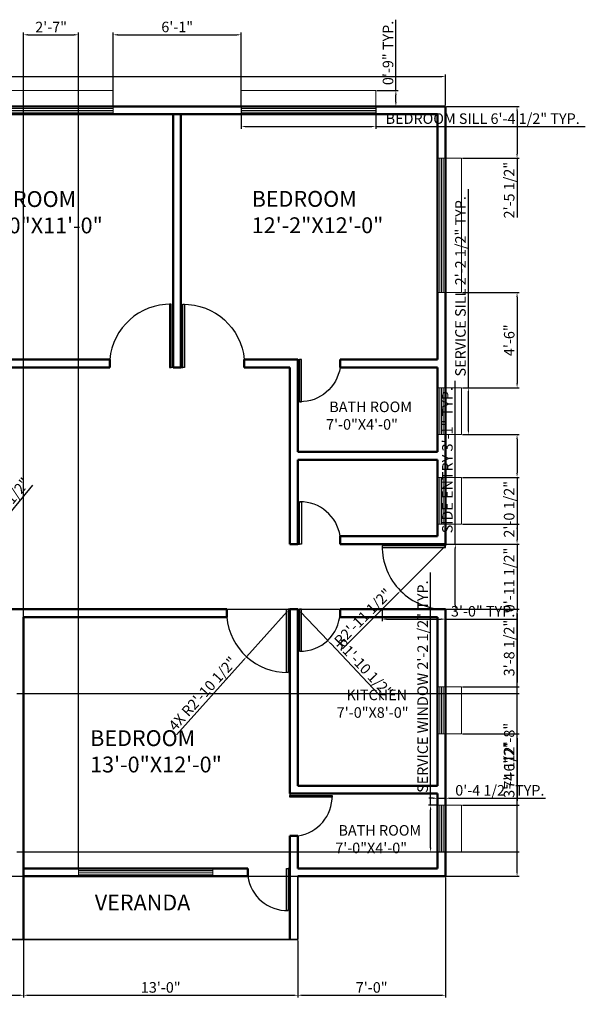
# Model space of a CAD drawing. Units: inches. Extents: x 2373 to 3112, y 1710 to 2270.
# Tile 2 of 2: x 2790 to 3112, y 1710 to 2270. Entities that reach past the tile are written whole.
import ezdxf

# ---------------------------------------------------------------- set-up
doc = ezdxf.new("R2010")
doc.units = ezdxf.units.IN
doc.layers.add('A-ANNO-DIMS', color=7, linetype='Continuous', lineweight=18)
doc.layers.add('A-AREA-IDEN', color=7, linetype='Continuous', lineweight=25)
for name, color, linetype, lineweight, true_color in [('A-DOOR', 114, 'Continuous', 25, 0x139b48), ('A-FLOR', 114, 'Continuous', 35, 0x139b48), ('A-GLAZ', 31, 'Continuous', 18, 0xfecc66), ('A-GLAZ-SILL', 30, 'Continuous', 18, 0xf8991e), ('A-WALL', 114, 'Continuous', 50, 0x139b48)]:
    doc.layers.add(name, color=color, linetype=linetype, lineweight=lineweight, true_color=true_color)
doc.styles.get("Standard").update_dxf_attribs({"font": 'arial.ttf'})
doc.dimstyles.new('ISO-25', dxfattribs={"dimtxt": 6, "dimasz": 2.5, "dimexe": 1.25, "dimexo": 0.625, "dimtad": 1, "dimdec": 1, "dimlunit": 3, "dimtxsty": 'Standard', "dimcen": 2.5, "dimadec": 0, "dimazin": 0, "dimtfac": 1, "dimtdec": 1, "dimtmove": 0, "dimatfit": 3, "dimfxl": 1, "dimarcsym": 0})

# ---------------------------------------------------------------- blocks, each defined once
blk = doc.blocks.new('*D2')
at = {"layer": 'A-ANNO-DIMS', "color": 0, "lineweight": -2, "transparency": 16777216}
for p, q in [((2426.36, 2221.72), (2426.36, 2239.32)), ((2428.86, 2238.07), (3029.86, 2238.07)), ((3032.36, 2221.72), (3032.36, 2239.32))]:
    blk.add_line(p, q, dxfattribs=at)
at = {"layer": 'A-ANNO-DIMS', "color": 0, "transparency": 16777216}
for points in [[(2428.86, 2238.48), (2428.86, 2237.65), (2426.36, 2238.07)], [(3029.86, 2238.48), (3029.86, 2237.65), (3032.36, 2238.07)]]:
    blk.add_solid(points, dxfattribs=at)
at = {"layer": 'Defpoints', "color": 0, "transparency": 16777216}
for p in [(3032.36, 2238.07), (2426.36, 2221.09), (3032.36, 2221.09)]:
    blk.add_point(p, dxfattribs=at)
at = {"layer": 'A-ANNO-DIMS', "color": 0, "transparency": 16777216, "insert": (2729.36, 2241.76), "char_height": 6, "attachment_point": 5}
blk.add_mtext('50\'-6"', dxfattribs=at)
blk = doc.blocks.new('DOOR-SWING-24IN')
for p, q in [((-2, -24), (-2, 0)), ((-2, 0), (-1, 0)), ((0, 0), (-1, 0)), ((-1, 0), (-1, -24)), ((-1, -24), (-2, -24))]:
    blk.add_line(p, q)
blk.add_arc((-1.5, -1.28), 22.73, 188.1552, 271.2605)
blk = doc.blocks.new('DOOR-SWING-36IN')
for p, q in [((-1, 36), (-2, 36)), ((-2, 36), (-2, 0)), ((-1, 0), (-1, 36)), ((-2, 0), (-1, 0)), ((0, 0), (-1, 0))]:
    blk.add_line(p, q)
blk.add_arc((-1.5, 1.36), 34.64, 89.173, 174.8014)
blk = doc.blocks.new('DOOR-SIDE-ENTRY-36IN')
for p, q in [((0, 0), (0, -1)), ((0, -1), (-36, -1)), ((-36, -1), (-36, -2)), ((-36, -2), (0, -2)), ((0, -2), (0, -1))]:
    blk.add_line(p, q)
blk.add_arc((-0.5, -1.5), 35.5, 179.1931, 270.8069)
blk = doc.blocks.new('WINDOW-BEDROOM')
for p, q in [((0, 0), (0, -4.5)), ((76.46, 0), (0, 0)), ((0, 0), (0, -2.25)), ((76.46, -4.5), (76.46, 0)), ((76.46, -1.25), (0, -1.25)), ((0, -1.25), (0, -2.25)), ((0, -2.25), (76.46, -2.25)), ((0, -2.25), (0, -3.25)), ((0, -3.25), (76.46, -3.25)), ((0, -4.5), (76.46, -4.5)), ((76.46, -2.25), (76.46, -1.25))]:
    blk.add_line(p, q)
blk = doc.blocks.new('WINDOW-SERVICE')
for p, q in [((0, 0), (0, -26.66)), ((4.5, 0), (0, 0)), ((1.25, 0), (1.25, -26.66)), ((2.25, 0), (2.25, -26.66)), ((3.25, -26.66), (3.25, 0)), ((4.5, -26.66), (4.5, 0)), ((4.5, -26.66), (4.5, 0)), ((0, -26.66), (4.5, -26.66))]:
    blk.add_line(p, q)
blk = doc.blocks.new('SILL-SERVICE')
for p, q in [((0, 0), (9, 0)), ((9, 0), (9, -26.66)), ((9, -26.66), (0, -26.66))]:
    blk.add_line(p, q)
blk = doc.blocks.new('SILL-BEDROOM')
for p, q in [((0, 0), (0, 9)), ((0, 9), (76.46, 9)), ((76.46, 9), (76.46, 0))]:
    blk.add_line(p, q)
blk = doc.blocks.new('*D16')
at = {"layer": 'A-ANNO-DIMS', "color": 0, "lineweight": -2, "transparency": 16777216}
for p, q in [((3037.93, 1972.09), (3037.93, 2065.02)), ((3032.99, 1972.09), (3039.18, 1972.09)), ((3037.93, 1937.46), (3037.93, 1969.59)), ((3032.99, 1934.96), (3039.18, 1934.96))]:
    blk.add_line(p, q, dxfattribs=at)
at = {"layer": 'A-ANNO-DIMS', "color": 0, "transparency": 16777216}
for points in [[(3037.52, 1969.59), (3038.35, 1969.59), (3037.93, 1972.09)], [(3037.52, 1937.46), (3038.35, 1937.46), (3037.93, 1934.96)]]:
    blk.add_solid(points, dxfattribs=at)
at = {"layer": 'Defpoints', "color": 0, "transparency": 16777216}
for p in [(3032.36, 1972.09), (3037.93, 1972.09), (3032.36, 1934.96)]:
    blk.add_point(p, dxfattribs=at)
at = {"layer": 'A-ANNO-DIMS', "color": 0, "transparency": 16777216, "insert": (3034.2, 2019.81), "char_height": 6, "attachment_point": 5, "rotation": 90}
blk.add_mtext('SIDE ENTRY 3\'-1" TYP.', dxfattribs=at)
blk = doc.blocks.new('*D17')
at = {"layer": 'A-ANNO-DIMS', "color": 0, "lineweight": -2, "transparency": 16777216}
for p, q in [((2996.23, 1934.33), (2996.23, 1928.14)), ((3032.36, 1934.33), (3032.36, 1928.14)), ((2998.73, 1929.39), (3029.86, 1929.39)), ((3032.36, 1929.39), (3072.68, 1929.39))]:
    blk.add_line(p, q, dxfattribs=at)
at = {"layer": 'A-ANNO-DIMS', "color": 0, "transparency": 16777216}
for points in [[(2998.73, 1929.81), (2998.73, 1928.97), (2996.23, 1929.39)], [(3029.86, 1929.81), (3029.86, 1928.97), (3032.36, 1929.39)]]:
    blk.add_solid(points, dxfattribs=at)
at = {"layer": 'Defpoints', "color": 0, "transparency": 16777216}
for p in [(2996.23, 1934.96), (3032.36, 1934.96), (3032.36, 1929.39)]:
    blk.add_point(p, dxfattribs=at)
at = {"layer": 'A-ANNO-DIMS', "color": 0, "transparency": 16777216, "insert": (3053.77, 1933.08), "char_height": 6, "attachment_point": 5}
blk.add_mtext('3\'-0" TYP.', dxfattribs=at)
blk = doc.blocks.new('*D20')
at = {"layer": 'A-ANNO-DIMS', "color": 0, "lineweight": -2, "transparency": 16777216}
for p, q in [((3023.86, 1823.48), (3023.86, 1955.99)), ((3027.24, 1823.48), (3022.61, 1823.48)), ((3023.86, 1799.32), (3023.86, 1820.98)), ((3027.24, 1796.82), (3022.61, 1796.82))]:
    blk.add_line(p, q, dxfattribs=at)
at = {"layer": 'A-ANNO-DIMS', "color": 0, "transparency": 16777216}
for points in [[(3023.45, 1820.98), (3024.28, 1820.98), (3023.86, 1823.48)], [(3023.45, 1799.32), (3024.28, 1799.32), (3023.86, 1796.82)]]:
    blk.add_solid(points, dxfattribs=at)
at = {"layer": 'Defpoints', "color": 0, "transparency": 16777216}
for p in [(3023.86, 1823.48), (3027.86, 1823.48), (3027.86, 1796.82)]:
    blk.add_point(p, dxfattribs=at)
at = {"layer": 'A-ANNO-DIMS', "color": 0, "transparency": 16777216, "insert": (3020.14, 1890.98), "char_height": 6, "attachment_point": 5, "rotation": 90}
blk.add_mtext('SERVICE WINDOW 2\'-2 1/2" TYP.', dxfattribs=at)
blk = doc.blocks.new('*D21')
at = {"layer": 'A-ANNO-DIMS', "color": 0, "lineweight": -2, "transparency": 16777216}
for p, q in [((3025.36, 1827.48), (3022.86, 1827.48)), ((3027.86, 1824.1), (3027.86, 1828.73)), ((3027.86, 1827.48), (3032.36, 1827.48)), ((3032.36, 1824.1), (3032.36, 1828.73)), ((3034.86, 1827.48), (3089.17, 1827.48))]:
    blk.add_line(p, q, dxfattribs=at)
at = {"layer": 'A-ANNO-DIMS', "color": 0, "transparency": 16777216}
for points in [[(3025.36, 1827.9), (3025.36, 1827.06), (3027.86, 1827.48)], [(3034.86, 1827.9), (3034.86, 1827.06), (3032.36, 1827.48)]]:
    blk.add_solid(points, dxfattribs=at)
at = {"layer": 'Defpoints', "color": 0, "transparency": 16777216}
for p in [(3032.36, 1827.48), (3027.86, 1823.48), (3032.36, 1823.48)]:
    blk.add_point(p, dxfattribs=at)
at = {"layer": 'A-ANNO-DIMS', "color": 0, "transparency": 16777216, "insert": (3063.27, 1831.21), "char_height": 6, "attachment_point": 5}
blk.add_mtext('0\'-4 1/2" TYP.', dxfattribs=at)
blk = doc.blocks.new('*D22')
at = {"layer": 'A-ANNO-DIMS', "color": 0, "lineweight": -2, "transparency": 16777216}
for p, q in [((3045.36, 2061), (3045.36, 2173.98)), ((3041.99, 2061), (3046.61, 2061)), ((3045.36, 2036.84), (3045.36, 2058.5)), ((3041.99, 2034.34), (3046.61, 2034.34))]:
    blk.add_line(p, q, dxfattribs=at)
at = {"layer": 'A-ANNO-DIMS', "color": 0, "transparency": 16777216}
for points in [[(3044.95, 2058.5), (3045.78, 2058.5), (3045.36, 2061)], [(3044.95, 2036.84), (3045.78, 2036.84), (3045.36, 2034.34)]]:
    blk.add_solid(points, dxfattribs=at)
at = {"layer": 'Defpoints', "color": 0, "transparency": 16777216}
for p in [(3041.36, 2061), (3045.36, 2061), (3041.36, 2034.34)]:
    blk.add_point(p, dxfattribs=at)
at = {"layer": 'A-ANNO-DIMS', "color": 0, "transparency": 16777216, "insert": (3041.64, 2118.74), "char_height": 6, "attachment_point": 5, "rotation": 90}
blk.add_mtext('SERVICE SILL 2\'-2 1/2" TYP.', dxfattribs=at)
blk = doc.blocks.new('*D24')
at = {"layer": 'A-ANNO-DIMS', "color": 0, "lineweight": -2, "transparency": 16777216}
for p, q in [((2916.18, 2220.47), (2916.18, 2208.38)), ((2992.64, 2220.47), (2992.64, 2208.38)), ((2918.68, 2209.63), (2990.14, 2209.63)), ((2992.64, 2209.63), (3111.89, 2209.63))]:
    blk.add_line(p, q, dxfattribs=at)
at = {"layer": 'A-ANNO-DIMS', "color": 0, "transparency": 16777216}
for points in [[(2918.68, 2210.04), (2918.68, 2209.21), (2916.18, 2209.63)], [(2990.14, 2210.04), (2990.14, 2209.21), (2992.64, 2209.63)]]:
    blk.add_solid(points, dxfattribs=at)
at = {"layer": 'Defpoints', "color": 0, "transparency": 16777216}
for p in [(2916.18, 2221.09), (2992.64, 2221.09), (2992.64, 2209.63)]:
    blk.add_point(p, dxfattribs=at)
at = {"layer": 'A-ANNO-DIMS', "color": 0, "transparency": 16777216, "insert": (3053.51, 2213.36), "char_height": 6, "attachment_point": 5}
blk.add_mtext('BEDROOM SILL 6\'-4 1/2" TYP.', dxfattribs=at)
blk = doc.blocks.new('*D25')
at = {"layer": 'A-ANNO-DIMS', "color": 0, "lineweight": -2, "transparency": 16777216}
for p, q in [((3004.11, 2230.09), (3004.11, 2270.42)), ((2993.26, 2230.09), (3005.36, 2230.09)), ((3004.11, 2223.59), (3004.11, 2227.59)), ((2993.26, 2221.09), (3005.36, 2221.09))]:
    blk.add_line(p, q, dxfattribs=at)
at = {"layer": 'A-ANNO-DIMS', "color": 0, "transparency": 16777216}
for points in [[(3003.69, 2227.59), (3004.53, 2227.59), (3004.11, 2230.09)], [(3003.69, 2223.59), (3004.53, 2223.59), (3004.11, 2221.09)]]:
    blk.add_solid(points, dxfattribs=at)
at = {"layer": 'Defpoints', "color": 0, "transparency": 16777216}
for p in [(2992.64, 2230.09), (3004.11, 2230.09), (2992.64, 2221.09)]:
    blk.add_point(p, dxfattribs=at)
at = {"layer": 'A-ANNO-DIMS', "color": 0, "transparency": 16777216, "insert": (3000.42, 2251.51), "char_height": 6, "attachment_point": 5, "rotation": 90}
blk.add_mtext('0\'-9" TYP.', dxfattribs=at)
blk = doc.blocks.new('*D31')
at = {"layer": 'A-ANNO-DIMS', "color": 0, "lineweight": -2, "transparency": 16777216}
for p, q in [((2670.86, 1746.47), (2670.86, 1714.14)), ((2792.36, 1746.47), (2792.36, 1714.14)), ((2673.36, 1715.39), (2789.86, 1715.39))]:
    blk.add_line(p, q, dxfattribs=at)
at = {"layer": 'A-ANNO-DIMS', "color": 0, "transparency": 16777216}
for points in [[(2673.36, 1715.81), (2673.36, 1714.97), (2670.86, 1715.39)], [(2789.86, 1715.81), (2789.86, 1714.97), (2792.36, 1715.39)]]:
    blk.add_solid(points, dxfattribs=at)
at = {"layer": 'Defpoints', "color": 0, "transparency": 16777216}
for p in [(2670.86, 1747.09), (2792.36, 1747.09), (2792.36, 1715.39)]:
    blk.add_point(p, dxfattribs=at)
at = {"layer": 'A-ANNO-DIMS', "color": 0, "transparency": 16777216, "insert": (2731.61, 1719.12), "char_height": 6, "attachment_point": 5}
blk.add_mtext('10\'-1 1/2"', dxfattribs=at)
blk = doc.blocks.new('*D32')
at = {"layer": 'A-ANNO-DIMS', "color": 0, "lineweight": -2, "transparency": 16777216}
for p, q in [((2792.36, 1746.47), (2792.36, 1714.14)), ((2948.36, 1746.47), (2948.36, 1714.14)), ((2794.86, 1715.39), (2945.86, 1715.39))]:
    blk.add_line(p, q, dxfattribs=at)
at = {"layer": 'A-ANNO-DIMS', "color": 0, "transparency": 16777216}
for points in [[(2794.86, 1715.81), (2794.86, 1714.97), (2792.36, 1715.39)], [(2945.86, 1715.81), (2945.86, 1714.97), (2948.36, 1715.39)]]:
    blk.add_solid(points, dxfattribs=at)
at = {"layer": 'Defpoints', "color": 0, "transparency": 16777216}
for p in [(2792.36, 1747.09), (2948.36, 1747.09), (2948.36, 1715.39)]:
    blk.add_point(p, dxfattribs=at)
at = {"layer": 'A-ANNO-DIMS', "color": 0, "transparency": 16777216, "insert": (2870.36, 1719.08), "char_height": 6, "attachment_point": 5}
blk.add_mtext('13\'-0"', dxfattribs=at)
blk = doc.blocks.new('*D33')
at = {"layer": 'A-ANNO-DIMS', "color": 0, "lineweight": -2, "transparency": 16777216}
for p, q in [((3032.36, 1782.47), (3032.36, 1714.14)), ((2948.36, 1746.47), (2948.36, 1714.14)), ((2950.86, 1715.39), (3029.86, 1715.39))]:
    blk.add_line(p, q, dxfattribs=at)
at = {"layer": 'A-ANNO-DIMS', "color": 0, "transparency": 16777216}
for points in [[(2950.86, 1715.81), (2950.86, 1714.97), (2948.36, 1715.39)], [(3029.86, 1715.81), (3029.86, 1714.97), (3032.36, 1715.39)]]:
    blk.add_solid(points, dxfattribs=at)
at = {"layer": 'Defpoints', "color": 0, "transparency": 16777216}
for p in [(3032.36, 1783.09), (2948.36, 1747.09), (3032.36, 1715.39)]:
    blk.add_point(p, dxfattribs=at)
at = {"layer": 'A-ANNO-DIMS', "color": 0, "transparency": 16777216, "insert": (2990.36, 1719.08), "char_height": 6, "attachment_point": 5}
blk.add_mtext('7\'-0"', dxfattribs=at)
blk = doc.blocks.new('*D34')
at = {"layer": 'A-ANNO-DIMS', "color": 0, "lineweight": -2, "transparency": 16777216}
for p, q in [((2555.99, 1935.09), (3074.32, 1935.09)), ((3073.07, 1785.59), (3073.07, 1932.59)), ((2571.63, 1783.09), (3074.32, 1783.09))]:
    blk.add_line(p, q, dxfattribs=at)
at = {"layer": 'A-ANNO-DIMS', "color": 0, "transparency": 16777216}
for points in [[(3072.65, 1932.59), (3073.49, 1932.59), (3073.07, 1935.09)], [(3072.65, 1785.59), (3073.49, 1785.59), (3073.07, 1783.09)]]:
    blk.add_solid(points, dxfattribs=at)
at = {"layer": 'Defpoints', "color": 0, "transparency": 16777216}
for p in [(2555.36, 1935.09), (3073.07, 1935.09), (2571, 1783.09)]:
    blk.add_point(p, dxfattribs=at)
at = {"layer": 'A-ANNO-DIMS', "color": 0, "transparency": 16777216, "insert": (3069.38, 1859.09), "char_height": 6, "attachment_point": 5, "rotation": 90}
blk.add_mtext('12\'-8"', dxfattribs=at)
blk = doc.blocks.new('*D38')
at = {"layer": 'A-ANNO-DIMS', "color": 0, "lineweight": -2, "transparency": 16777216}
for p, q in [((2843.26, 2221.72), (2843.26, 2263.07)), ((2845.76, 2261.82), (2913.68, 2261.82)), ((2916.18, 2221.72), (2916.18, 2263.07))]:
    blk.add_line(p, q, dxfattribs=at)
at = {"layer": 'A-ANNO-DIMS', "color": 0, "transparency": 16777216}
for points in [[(2845.76, 2262.24), (2845.76, 2261.4), (2843.26, 2261.82)], [(2913.68, 2262.24), (2913.68, 2261.4), (2916.18, 2261.82)]]:
    blk.add_solid(points, dxfattribs=at)
at = {"layer": 'Defpoints', "color": 0, "transparency": 16777216}
for p in [(2916.18, 2261.82), (2843.26, 2221.09), (2916.18, 2221.09)]:
    blk.add_point(p, dxfattribs=at)
at = {"layer": 'A-ANNO-DIMS', "color": 0, "transparency": 16777216, "insert": (2879.72, 2265.51), "char_height": 6, "attachment_point": 5}
blk.add_mtext('6\'-1"', dxfattribs=at)
blk = doc.blocks.new('*D39')
at = {"layer": 'A-ANNO-DIMS', "color": 0, "lineweight": -2, "transparency": 16777216}
for p, q in [((3032.99, 2221.09), (3074.32, 2221.09)), ((3073.07, 2218.59), (3073.07, 2194.08)), ((3041.99, 2191.58), (3074.32, 2191.58)), ((3073.07, 2191.58), (3073.07, 2157.79))]:
    blk.add_line(p, q, dxfattribs=at)
at = {"layer": 'A-ANNO-DIMS', "color": 0, "transparency": 16777216}
for points in [[(3072.65, 2218.59), (3073.49, 2218.59), (3073.07, 2221.09)], [(3072.65, 2194.08), (3073.49, 2194.08), (3073.07, 2191.58)]]:
    blk.add_solid(points, dxfattribs=at)
at = {"layer": 'Defpoints', "color": 0, "transparency": 16777216}
for p in [(3032.36, 2221.09), (3041.36, 2191.58), (3073.07, 2191.58)]:
    blk.add_point(p, dxfattribs=at)
at = {"layer": 'A-ANNO-DIMS', "color": 0, "transparency": 16777216, "insert": (3069.34, 2173.44), "char_height": 6, "attachment_point": 5, "rotation": 90}
blk.add_mtext('2\'-5 1/2"', dxfattribs=at)
blk = doc.blocks.new('*D40')
at = {"layer": 'A-ANNO-DIMS', "color": 0, "lineweight": -2, "transparency": 16777216}
for p, q in [((3041.99, 2115.12), (3074.32, 2115.12)), ((3073.07, 2112.62), (3073.07, 2063.5)), ((3041.99, 2061), (3074.32, 2061))]:
    blk.add_line(p, q, dxfattribs=at)
at = {"layer": 'A-ANNO-DIMS', "color": 0, "transparency": 16777216}
for points in [[(3072.65, 2112.62), (3073.49, 2112.62), (3073.07, 2115.12)], [(3072.65, 2063.5), (3073.49, 2063.5), (3073.07, 2061)]]:
    blk.add_solid(points, dxfattribs=at)
at = {"layer": 'Defpoints', "color": 0, "transparency": 16777216}
for p in [(3041.36, 2115.12), (3041.36, 2061), (3073.07, 2061)]:
    blk.add_point(p, dxfattribs=at)
at = {"layer": 'A-ANNO-DIMS', "color": 0, "transparency": 16777216, "insert": (3069.38, 2088.06), "char_height": 6, "attachment_point": 5, "rotation": 90}
blk.add_mtext('4\'-6"', dxfattribs=at)
blk = doc.blocks.new('*D41')
at = {"layer": 'A-ANNO-DIMS', "color": 0, "lineweight": -2, "transparency": 16777216}
for p, q in [((3041.99, 2034.34), (3074.32, 2034.34)), ((3073.07, 2031.84), (3073.07, 2012.53)), ((3041.99, 2010.03), (3074.32, 2010.03)), ((3073.07, 2010.03), (3073.07, 1976.25))]:
    blk.add_line(p, q, dxfattribs=at)
at = {"layer": 'A-ANNO-DIMS', "color": 0, "transparency": 16777216}
for points in [[(3072.65, 2031.84), (3073.49, 2031.84), (3073.07, 2034.34)], [(3072.65, 2012.53), (3073.49, 2012.53), (3073.07, 2010.03)]]:
    blk.add_solid(points, dxfattribs=at)
at = {"layer": 'Defpoints', "color": 0, "transparency": 16777216}
for p in [(3041.36, 2034.34), (3041.36, 2010.03), (3073.07, 2010.03)]:
    blk.add_point(p, dxfattribs=at)
at = {"layer": 'A-ANNO-DIMS', "color": 0, "transparency": 16777216, "insert": (3069.34, 1991.89), "char_height": 6, "attachment_point": 5, "rotation": 90}
blk.add_mtext('2\'-0 1/2"', dxfattribs=at)
blk = doc.blocks.new('*D42')
at = {"layer": 'A-ANNO-DIMS', "color": 0, "lineweight": -2, "transparency": 16777216}
for p, q in [((3041.99, 1983.37), (3074.32, 1983.37)), ((3073.07, 1980.87), (3073.07, 1974.59)), ((3032.99, 1972.09), (3074.32, 1972.09)), ((3073.07, 1972.09), (3073.07, 1933.75))]:
    blk.add_line(p, q, dxfattribs=at)
at = {"layer": 'A-ANNO-DIMS', "color": 0, "transparency": 16777216}
for points in [[(3072.65, 1980.87), (3073.49, 1980.87), (3073.07, 1983.37)], [(3072.65, 1974.59), (3073.49, 1974.59), (3073.07, 1972.09)]]:
    blk.add_solid(points, dxfattribs=at)
at = {"layer": 'Defpoints', "color": 0, "transparency": 16777216}
for p in [(3041.36, 1983.37), (3032.36, 1972.09), (3073.07, 1972.09)]:
    blk.add_point(p, dxfattribs=at)
at = {"layer": 'A-ANNO-DIMS', "color": 0, "transparency": 16777216, "insert": (3069.34, 1951.67), "char_height": 6, "attachment_point": 5, "rotation": 90}
blk.add_mtext('0\'-11 1/2"', dxfattribs=at)
blk = doc.blocks.new('*D43')
at = {"layer": 'A-ANNO-DIMS', "color": 0, "lineweight": -2, "transparency": 16777216}
for p, q in [((3032.99, 1935.09), (3074.32, 1935.09)), ((3073.07, 1932.59), (3073.07, 1893.29)), ((3041.99, 1890.79), (3074.32, 1890.79))]:
    blk.add_line(p, q, dxfattribs=at)
at = {"layer": 'A-ANNO-DIMS', "color": 0, "transparency": 16777216}
for points in [[(3072.65, 1932.59), (3073.49, 1932.59), (3073.07, 1935.09)], [(3072.65, 1893.29), (3073.49, 1893.29), (3073.07, 1890.79)]]:
    blk.add_solid(points, dxfattribs=at)
at = {"layer": 'Defpoints', "color": 0, "transparency": 16777216}
for p in [(3032.36, 1935.09), (3041.36, 1890.79), (3073.07, 1890.79)]:
    blk.add_point(p, dxfattribs=at)
at = {"layer": 'A-ANNO-DIMS', "color": 0, "transparency": 16777216, "insert": (3069.34, 1912.94), "char_height": 6, "attachment_point": 5, "rotation": 90}
blk.add_mtext('3\'-8 1/2"', dxfattribs=at)
blk = doc.blocks.new('*D44')
at = {"layer": 'A-ANNO-DIMS', "color": 0, "lineweight": -2, "transparency": 16777216}
for p, q in [((3041.99, 1864.13), (3074.32, 1864.13)), ((3073.07, 1861.63), (3073.07, 1825.98)), ((3041.99, 1823.48), (3074.32, 1823.48))]:
    blk.add_line(p, q, dxfattribs=at)
at = {"layer": 'A-ANNO-DIMS', "color": 0, "transparency": 16777216}
for points in [[(3072.65, 1861.63), (3073.49, 1861.63), (3073.07, 1864.13)], [(3072.65, 1825.98), (3073.49, 1825.98), (3073.07, 1823.48)]]:
    blk.add_solid(points, dxfattribs=at)
at = {"layer": 'Defpoints', "color": 0, "transparency": 16777216}
for p in [(3041.36, 1864.13), (3041.36, 1823.48), (3073.07, 1823.48)]:
    blk.add_point(p, dxfattribs=at)
at = {"layer": 'A-ANNO-DIMS', "color": 0, "transparency": 16777216, "insert": (3069.34, 1843.8), "char_height": 6, "attachment_point": 5, "rotation": 90}
blk.add_mtext('3\'-4 1/2"', dxfattribs=at)
blk = doc.blocks.new('*D49')
at = {"layer": 'A-ANNO-DIMS', "color": 0, "lineweight": -2, "transparency": 16777216}
for p, q in [((2792.36, 1788.22), (2792.36, 2263.07)), ((2794.86, 2261.82), (2821.09, 2261.82)), ((2823.59, 1788.22), (2823.59, 2263.07))]:
    blk.add_line(p, q, dxfattribs=at)
at = {"layer": 'A-ANNO-DIMS', "color": 0, "transparency": 16777216}
for points in [[(2794.86, 2262.24), (2794.86, 2261.4), (2792.36, 2261.82)], [(2821.09, 2262.24), (2821.09, 2261.4), (2823.59, 2261.82)]]:
    blk.add_solid(points, dxfattribs=at)
at = {"layer": 'Defpoints', "color": 0, "transparency": 16777216}
for p in [(2823.59, 2261.82), (2792.36, 1787.59), (2823.59, 1787.59)]:
    blk.add_point(p, dxfattribs=at)
at = {"layer": 'A-ANNO-DIMS', "color": 0, "transparency": 16777216, "insert": (2807.98, 2265.46), "char_height": 6, "attachment_point": 5}
blk.add_mtext('2\'-7"', dxfattribs=at)
blk = doc.blocks.new('*D52')
at = {"layer": 'A-ANNO-DIMS', "color": 0, "lineweight": -2, "transparency": 16777216}
for p, q in [((2788.49, 1887.04), (3074.32, 1887.04)), ((3073.07, 1799.54), (3073.07, 1884.54)), ((2788.49, 1797.04), (3074.32, 1797.04))]:
    blk.add_line(p, q, dxfattribs=at)
at = {"layer": 'A-ANNO-DIMS', "color": 0, "transparency": 16777216}
for points in [[(3072.65, 1884.54), (3073.49, 1884.54), (3073.07, 1887.04)], [(3072.65, 1799.54), (3073.49, 1799.54), (3073.07, 1797.04)]]:
    blk.add_solid(points, dxfattribs=at)
at = {"layer": 'Defpoints', "color": 0, "transparency": 16777216}
for p in [(2787.86, 1887.04), (3073.07, 1887.04), (2787.86, 1797.04)]:
    blk.add_point(p, dxfattribs=at)
at = {"layer": 'A-ANNO-DIMS', "color": 0, "transparency": 16777216, "insert": (3069.38, 1842.04), "char_height": 6, "attachment_point": 5, "rotation": 90}
blk.add_mtext('7\'-6"', dxfattribs=at)
blk = doc.blocks.new('*D53')
at = {"layer": 'A-ANNO-DIMS', "color": 0, "lineweight": -2, "transparency": 16777216}
for p, q in [((2797.34, 2005.57), (2766.87, 1968.4)), ((2731.36, 1925.09), (2765.28, 1966.47))]:
    blk.add_line(p, q, dxfattribs=at)
at = {"layer": 'A-ANNO-DIMS', "color": 0, "transparency": 16777216}
blk.add_solid([(2766.55, 1968.67), (2767.19, 1968.14), (2765.28, 1966.47)], dxfattribs=at)
at = {"layer": 'Defpoints', "color": 0, "transparency": 16777216}
for p in [(2765.28, 1966.47), (2731.36, 1925.09)]:
    blk.add_point(p, dxfattribs=at)
at = {"layer": 'A-ANNO-DIMS', "color": 0, "transparency": 16777216, "insert": (2782.75, 1993.66), "char_height": 6, "attachment_point": 5, "rotation": 50.654}
blk.add_mtext('R4\'-5 1/2"', dxfattribs=at)
blk = doc.blocks.new('*D55')
at = {"layer": 'A-ANNO-DIMS', "color": 0, "lineweight": -2, "transparency": 16777216}
for p, q in [((3031.86, 1970.59), (3006.76, 1945.49)), ((2973.82, 1912.55), (3004.99, 1943.72))]:
    blk.add_line(p, q, dxfattribs=at)
at = {"layer": 'A-ANNO-DIMS', "color": 0, "transparency": 16777216}
blk.add_solid([(3004.7, 1944.02), (3005.29, 1943.43), (3006.76, 1945.49)], dxfattribs=at)
at = {"layer": 'Defpoints', "color": 0, "transparency": 16777216}
for p in [(3031.86, 1970.59), (3006.76, 1945.49)]:
    blk.add_point(p, dxfattribs=at)
at = {"layer": 'A-ANNO-DIMS', "color": 0, "transparency": 16777216, "insert": (2985.89, 1929.89), "char_height": 6, "attachment_point": 5, "rotation": 45.0001}
blk.add_mtext('R2\'-11 1/2"', dxfattribs=at)
blk = doc.blocks.new('*D56')
at = {"layer": 'A-ANNO-DIMS', "color": 0, "lineweight": -2, "transparency": 16777216}
for p, q in [((2942.36, 1933.73), (2919.19, 1907.98)), ((2879.24, 1863.6), (2917.52, 1906.13))]:
    blk.add_line(p, q, dxfattribs=at)
at = {"layer": 'A-ANNO-DIMS', "color": 0, "transparency": 16777216}
blk.add_solid([(2917.21, 1906.4), (2917.83, 1905.85), (2919.19, 1907.98)], dxfattribs=at)
at = {"layer": 'Defpoints', "color": 0, "transparency": 16777216}
for p in [(2942.36, 1933.73), (2919.19, 1907.98)]:
    blk.add_point(p, dxfattribs=at)
at = {"layer": 'A-ANNO-DIMS', "color": 0, "transparency": 16777216, "insert": (2894.77, 1886.43), "char_height": 6, "attachment_point": 5, "rotation": 48.0129}
blk.add_mtext('4X R2\'-10 1/2"', dxfattribs=at)
blk = doc.blocks.new('*D58')
at = {"layer": 'A-ANNO-DIMS', "color": 0, "lineweight": -2, "transparency": 16777216}
for p, q in [((2949.86, 1933.6), (2965.33, 1917.24)), ((2997.34, 1883.4), (2967.05, 1915.43))]:
    blk.add_line(p, q, dxfattribs=at)
at = {"layer": 'A-ANNO-DIMS', "color": 0, "transparency": 16777216}
blk.add_solid([(2967.35, 1915.71), (2966.75, 1915.14), (2965.33, 1917.24)], dxfattribs=at)
at = {"layer": 'Defpoints', "color": 0, "transparency": 16777216}
for p in [(2949.86, 1933.6), (2965.33, 1917.24)]:
    blk.add_point(p, dxfattribs=at)
at = {"layer": 'A-ANNO-DIMS', "color": 0, "transparency": 16777216, "insert": (2985.76, 1901.07), "char_height": 6, "attachment_point": 5, "rotation": 313.4012}
blk.add_mtext('R1\'-10 1/2"', dxfattribs=at)

msp = doc.modelspace()

# ---------------------------------------------------------------- linework, layer by layer
at = {"layer": 'A-DOOR'}
for p, q in [((2941.86, 1899.09), (2941.86, 1935.09)), ((2941.86, 1935.09), (2943.36, 1935.09)), ((2943.86, 1935.09), (2942.86, 1935.09)), ((2942.86, 1935.09), (2942.86, 1899.09)), ((2948.36, 1935.09), (2949.36, 1935.09)), ((2949.36, 1935.09), (2949.36, 1911.09)), ((2950.36, 1935.09), (2949.36, 1935.09)), ((2949.36, 1935.09), (2949.36, 1911.09)), ((2950.36, 1911.09), (2950.36, 1935.09)), ((2949.36, 1911.09), (2950.36, 1911.09)), ((2942.86, 1899.09), (2941.86, 1899.09))]:
    msp.add_line(p, q, dxfattribs=at)
for centre, radius, start, end in [((2949.86, 1933.6), 22.51, 268.7274, 358.0726), ((2942.36, 1933.73), 34.64, 185.1986, 270.827)]:
    msp.add_arc(centre, radius, start, end, dxfattribs=at)
at = {"layer": 'A-FLOR'}
for p, q in [((2948.36, 1747.09), (2948.36, 1783.09)), ((2514.86, 1747.09), (2948.36, 1747.09))]:
    msp.add_line(p, q, dxfattribs=at)
at = {"layer": 'A-GLAZ-SILL'}
for p, q in [((3032.36, 2191.58), (3041.36, 2191.58)), ((3041.36, 2191.58), (3041.36, 2115.12)), ((3041.36, 2115.12), (3030.61, 2115.12))]:
    msp.add_line(p, q, dxfattribs=at)
at = {"layer": 'A-WALL'}
for p, q in [((2426.36, 2221.09), (3032.36, 2221.09)), ((3032.36, 2221.09), (3032.36, 1972.09)), ((2430.86, 2216.59), (3027.86, 2216.59)), ((2877.36, 2216.59), (2877.36, 2072.59)), ((2881.86, 2216.59), (2881.86, 2072.59)), ((3027.86, 2216.59), (3027.86, 2077.09)), ((2729.86, 2077.09), (2841.36, 2077.09)), ((2841.36, 2072.59), (2841.36, 2077.09)), ((2917.86, 2072.59), (2917.86, 2077.09)), ((2917.86, 2077.09), (2948.36, 2077.09)), ((2948.36, 2072.59), (2948.36, 2077.09)), ((2972.36, 2077.09), (2972.36, 2072.59)), ((2972.36, 2077.09), (3027.86, 2077.09)), ((2729.86, 2072.59), (2841.36, 2072.59)), ((2877.36, 2072.59), (2881.86, 2072.59)), ((2917.86, 2072.59), (2943.86, 2072.59)), ((2943.86, 2072.59), (2943.86, 1972.09)), ((2948.36, 2072.59), (2948.36, 2024.59)), ((2972.36, 2072.59), (3027.86, 2072.59)), ((3027.86, 2072.59), (3027.86, 2024.59)), ((2948.36, 2024.59), (3027.86, 2024.59)), ((2948.36, 2020.09), (3027.86, 2020.09)), ((2948.36, 2020.09), (2948.36, 1972.09)), ((3027.86, 2020.09), (3027.86, 1976.59)), ((2943.86, 1972.09), (2948.36, 1972.09)), ((2972.36, 1972.09), (2972.36, 1976.59)), ((2972.36, 1976.59), (3027.86, 1976.59)), ((2972.36, 1972.09), (3032.36, 1972.09)), ((2783.92, 1935.09), (2907.86, 1935.09)), ((2907.86, 1930.59), (2907.86, 1935.09)), ((2943.86, 1935.09), (2943.86, 1830.09)), ((2943.86, 1935.09), (2948.36, 1935.09)), ((2948.36, 1935.09), (2948.36, 1834.59)), ((2972.36, 1930.59), (2972.36, 1935.09)), ((2972.36, 1935.09), (3032.36, 1935.09)), ((3032.36, 1935.09), (3032.36, 1783.09)), ((2792.36, 1930.59), (2792.36, 1747.09)), ((2792.36, 1930.59), (2907.86, 1930.59)), ((2972.36, 1930.59), (3027.86, 1930.59)), ((3027.86, 1930.59), (3027.86, 1834.59)), ((2948.36, 1834.59), (3027.86, 1834.59)), ((2943.86, 1830.09), (3027.86, 1830.09)), ((3027.86, 1830.09), (3027.86, 1787.59)), ((2948.36, 1806.09), (2943.86, 1806.09)), ((2943.86, 1806.09), (2943.86, 1747.09)), ((2948.36, 1806.09), (2948.36, 1787.59)), ((2919.86, 1787.59), (2792.36, 1787.59)), ((2919.86, 1783.09), (2919.86, 1787.59)), ((3027.86, 1787.59), (2948.36, 1787.59)), ((2919.86, 1783.09), (2792.36, 1783.09)), ((3032.36, 1783.09), (2948.36, 1783.09))]:
    msp.add_line(p, q, dxfattribs=at)

# ---------------------------------------------------------------- block references
at = {"layer": 'A-DOOR'}
for name, p in [('DOOR-SWING-36IN', (2877.36, 2072.59)), ('DOOR-SIDE-ENTRY-36IN', (3032.36, 1972.09)), ('DOOR-SWING-24IN', (2943.86, 1787.59))]:
    msp.add_blockref(name, p, dxfattribs=at)
at = {"layer": 'A-DOOR', "extrusion": (0, 0, -1), "zscale": -1}
for name, p in [('DOOR-SWING-36IN', (-2881.86, 2072.59)), ('DOOR-SWING-24IN', (-2948.36, 2077.09))]:
    msp.add_blockref(name, p, dxfattribs=at)
at = {"layer": 'A-DOOR'}
for p, rotation in [((2948.36, 1972.09), 180), ((2943.86, 1830.09), 89.99999999999854)]:
    msp.add_blockref('DOOR-SWING-24IN', p, dxfattribs=dict(at, rotation=rotation))
at = {"layer": 'A-GLAZ'}
for name, p in [('WINDOW-BEDROOM', (2766.8, 2221.09)), ('WINDOW-BEDROOM', (2916.18, 2221.09)), ('WINDOW-SERVICE', (3027.86, 2061)), ('WINDOW-SERVICE', (3027.86, 2010.03)), ('WINDOW-SERVICE', (3027.86, 1890.79)), ('WINDOW-SERVICE', (3027.86, 1823.48))]:
    msp.add_blockref(name, p, dxfattribs=at)
for p, rotation in [((3027.86, 2115.12), 90.0000000000013), ((2900.05, 1783.09), 180)]:
    msp.add_blockref('WINDOW-BEDROOM', p, dxfattribs=dict(at, rotation=rotation))
at = {"layer": 'A-GLAZ-SILL'}
for name, p in [('SILL-BEDROOM', (2766.8, 2221.09)), ('SILL-BEDROOM', (2916.18, 2221.09)), ('SILL-SERVICE', (3032.36, 2061)), ('SILL-SERVICE', (3032.36, 2010.03)), ('SILL-SERVICE', (3032.36, 1890.79)), ('SILL-SERVICE', (3032.36, 1823.48))]:
    msp.add_blockref(name, p, dxfattribs=at)

# ---------------------------------------------------------------- texts
at = {"layer": 'A-AREA-IDEN', "attachment_point": 1}
for s, insert, char_height in [('BEDROOM\\P12\'-0"X11\'-0"', (2762.49, 2172.87), 9), ('BEDROOM\\P12\'-2"X12\'-0"', (2922.1, 2172.98), 9), (' BATH ROOM\\P   7\'-0"X4\'-0"', (2964.41, 2053.16), 6), ('   KITCHEN\\P   7\'-0"X8\'-0"', (2970.48, 1889.26), 6), ('BEDROOM\\P13\'-0"X12\'-0"', (2830.21, 1866.17), 9), (' BATH ROOM\\P   7\'-0"X4\'-0"', (2969.63, 1812.21), 6), ('VERANDA', (2832.83, 1772.7), 9)]:
    msp.add_mtext(s, dxfattribs=dict(at, insert=insert, char_height=char_height))

# ---------------------------------------------------------------- dimensions: what is measured, and where the dimension line sits
at = {"layer": 'A-ANNO-DIMS'}
for base, p1, p2, override, picture, middle in [((2823.59, 2261.82), (2792.36, 1787.59), (2823.59, 1787.59), {"dimdec": 1, "dimlfac": 1, "dimrnd": 0, "dimzin": 1, "dimdsep": 46, "dimlunit": 4, "dimfrac": 2}, '*D49', (2807.98, 2265.46)), ((2916.18, 2261.82), (2843.26, 2221.09), (2916.18, 2221.09), {"dimdec": 1, "dimlfac": 1, "dimrnd": 0, "dimzin": 1, "dimdsep": 46, "dimlunit": 4, "dimfrac": 2}, '*D38', (2879.72, 2265.51)), ((3032.36, 2238.07), (2426.36, 2221.09), (3032.36, 2221.09), {"dimclrd": 0, "dimclre": 0, "dimclrt": 0}, '*D2', (2729.36, 2241.76)), ((3032.36, 1715.39), (2948.36, 1747.09), (3032.36, 1783.09), {"dimdec": 1, "dimlfac": 1, "dimrnd": 0, "dimzin": 1, "dimdsep": 46, "dimlunit": 4, "dimfrac": 2}, '*D33', (2990.36, 1719.08)), ((2792.36, 1715.39), (2670.86, 1747.09), (2792.36, 1747.09), {"dimdec": 1, "dimlfac": 1, "dimrnd": 0, "dimzin": 1, "dimdsep": 46, "dimlunit": 4, "dimfrac": 2}, '*D31', (2731.61, 1719.12)), ((2948.36, 1715.39), (2792.36, 1747.09), (2948.36, 1747.09), {"dimdec": 1, "dimlfac": 1, "dimrnd": 0, "dimzin": 1, "dimdsep": 46, "dimlunit": 4, "dimfrac": 2}, '*D32', (2870.36, 1719.08))]:
    dim = msp.add_linear_dim(base=base, p1=p1, p2=p2, dimstyle='ISO-25', override=override, dxfattribs=at)
    dim.commit()
    dim.dimension.update_dxf_attribs({"geometry": picture, "text_midpoint": middle})
for base, p1, p2, text, picture, middle in [((3004.11, 2230.09), (2992.64, 2221.09), (2992.64, 2230.09), '<> TYP.', '*D25', (3000.42, 2251.51)), ((3045.36, 2061), (3041.36, 2034.34), (3041.36, 2061), 'SERVICE SILL <> TYP.', '*D22', (3041.64, 2118.74)), ((3037.93, 1972.09), (3032.36, 1934.96), (3032.36, 1972.09), 'SIDE ENTRY <> TYP.', '*D16', (3034.2, 2019.81)), ((3023.86, 1823.48), (3027.86, 1796.82), (3027.86, 1823.48), 'SERVICE WINDOW <> TYP.', '*D20', (3020.14, 1890.98))]:
    dim = msp.add_linear_dim(base=base, p1=p1, p2=p2, angle=90, text=text, dimstyle='ISO-25', override={"dimdec": 1, "dimlfac": 1, "dimrnd": 0, "dimzin": 1, "dimdsep": 46, "dimlunit": 4, "dimfrac": 2}, dxfattribs=at)
    dim.commit()
    dim.dimension.update_dxf_attribs({"geometry": picture, "text_midpoint": middle})
for base, p1, p2, text, picture, middle in [((2992.64, 2209.63), (2916.18, 2221.09), (2992.64, 2221.09), 'BEDROOM SILL <> TYP.', '*D24', (3053.51, 2213.36)), ((3032.36, 1929.39), (2996.23, 1934.96), (3032.36, 1934.96), '<> TYP.', '*D17', (3053.77, 1933.08)), ((3032.36, 1827.48), (3027.86, 1823.48), (3032.36, 1823.48), '<> TYP.', '*D21', (3063.27, 1831.21))]:
    dim = msp.add_linear_dim(base=base, p1=p1, p2=p2, text=text, dimstyle='ISO-25', override={"dimdec": 1, "dimlfac": 1, "dimrnd": 0, "dimzin": 1, "dimdsep": 46, "dimlunit": 4, "dimfrac": 2}, dxfattribs=at)
    dim.commit()
    dim.dimension.update_dxf_attribs({"geometry": picture, "text_midpoint": middle})
for base, p1, p2, picture, middle in [((3073.07, 2191.58), (3032.36, 2221.09), (3041.36, 2191.58), '*D39', (3069.34, 2173.44)), ((3073.07, 2061), (3041.36, 2115.12), (3041.36, 2061), '*D40', (3069.38, 2088.06)), ((3073.07, 2010.03), (3041.36, 2034.34), (3041.36, 2010.03), '*D41', (3069.34, 1991.89)), ((3073.07, 1972.09), (3041.36, 1983.37), (3032.36, 1972.09), '*D42', (3069.34, 1951.67)), ((3073.07, 1935.09), (2571, 1783.09), (2555.36, 1935.09), '*D34', (3069.38, 1859.09)), ((3073.07, 1890.79), (3032.36, 1935.09), (3041.36, 1890.79), '*D43', (3069.34, 1912.94)), ((3073.07, 1887.04), (2787.86, 1797.04), (2787.86, 1887.04), '*D52', (3069.38, 1842.04)), ((3073.0685, 1823.4795), (3041.3635, 1864.1269), (3041.3635, 1823.4795), '*D44', (3069.3391, 1843.8032))]:
    dim = msp.add_linear_dim(base=base, p1=p1, p2=p2, angle=90, dimstyle='ISO-25', override={"dimdec": 1, "dimlfac": 1, "dimrnd": 0, "dimzin": 1, "dimdsep": 46, "dimlunit": 4, "dimfrac": 2}, dxfattribs=at)
    dim.commit()
    dim.dimension.update_dxf_attribs({"geometry": picture, "text_midpoint": middle})
dim = msp.add_radius_dim(center=(2731.36, 1925.09), mpoint=(2765.28, 1966.47), dimstyle='ISO-25', override={"dimdec": 1, "dimlfac": 1, "dimrnd": 0, "dimzin": 1, "dimdsep": 46, "dimlunit": 4, "dimfrac": 2}, dxfattribs=at)
dim.commit()
dim.dimension.update_dxf_attribs({"geometry": '*D53', "text_midpoint": (2785.64, 1991.29), "dimtype": 164})
for center, mpoint, picture, middle in [((3031.86, 1970.59), (3006.76, 1945.49), '*D55', (2985.89, 1929.89)), ((2949.86, 1933.6), (2965.33, 1917.24), '*D58', (2985.76, 1901.07))]:
    dim = msp.add_radius_dim(center=center, mpoint=mpoint, dimstyle='ISO-25', override={"dimdec": 1, "dimlfac": 1, "dimrnd": 0, "dimzin": 1, "dimdsep": 46, "dimlunit": 4, "dimfrac": 2}, dxfattribs=at)
    dim.commit()
    dim.dimension.update_dxf_attribs({"geometry": picture, "text_midpoint": middle})
dim = msp.add_radius_dim(center=(2942.36, 1933.73), mpoint=(2919.19, 1907.98), text='4X <>', dimstyle='ISO-25', override={"dimdec": 1, "dimlfac": 1, "dimrnd": 0, "dimzin": 1, "dimdsep": 46, "dimlunit": 4, "dimfrac": 2}, dxfattribs=at)
dim.commit()
dim.dimension.update_dxf_attribs({"geometry": '*D56', "text_midpoint": (2894.77, 1886.43)})

doc.saveas('drawing.dxf')
